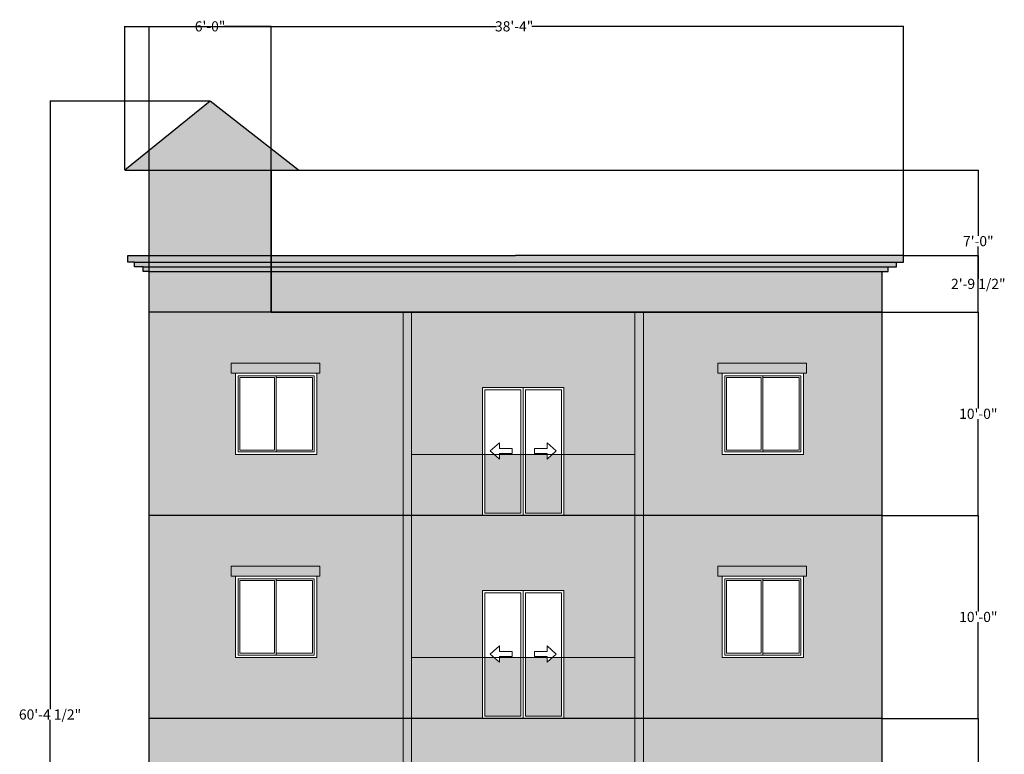
# Model space of a CAD drawing. Units: inches. Extents: x -113 to 5399, y -1393 to 3302.
# Tile 21 of 40: x 3613 to 4195, y -941 to -507. Entities that reach past the tile are written whole.
import ezdxf

# ---------------------------------------------------------------- set-up
doc = ezdxf.new("R2010")
doc.units = ezdxf.units.IN
doc.header["$MEASUREMENT"] = 0
for name, color, linetype, lineweight in [('A-ANNO-DIMS', 254, 'Continuous', 18), ('A-Door', 150, 'Continuous', 18), ('A-ELEV', 7, 'Continuous', 25), ('A-ELEV-GLAZ', 150, 'Continuous', 18), ('A-ELEV-RAIL', 7, 'Continuous', 18), ('A-ELEV-TRIM', 7, 'Continuous', 18), ('A-ELEV-TRIM-PATT', 7, 'Continuous', 13), ('A-ROOF', 7, 'Continuous', 25), ('A-ROOF-CORN-PATT', 3, 'Continuous', 13)]:
    doc.layers.add(name, color=color, linetype=linetype, lineweight=lineweight)
for name, color, linetype, lineweight, true_color in [('A-ELEV-RAIL-PATT', 9, 'Continuous', 13, 0xc7c8ca), ('A-ELEV-WALL-PATT', 241, 'Continuous', 13, 0xf7abae), ('A-ROOF-PATT', 251, 'Continuous', 13, 0x636466)]:
    doc.layers.add(name, color=color, linetype=linetype, lineweight=lineweight, true_color=true_color)
doc.styles.get("Standard").update_dxf_attribs({"font": 'arial.ttf'})
doc.dimstyles.get("Standard").update_dxf_attribs({"dimtxt": 6, "dimasz": 0.18, "dimexe": 0.18, "dimexo": 0.0625, "dimgap": 0.09, "dimtad": 0, "dimtih": 1, "dimtoh": 1, "dimdec": 1, "dimzin": 0, "dimdsep": 46, "dimlunit": 4, "dimtxsty": 'Standard', "dimblk": 'ARCHTICK', "dimcen": 0.09, "dimadec": 0, "dimazin": 0, "dimtfac": 1, "dimtdec": 1, "dimtofl": 0, "dimtmove": 0, "dimatfit": 3, "dimfxl": 1, "dimtolj": 1, "dimtzin": 0, "dimarcsym": 0})

# ---------------------------------------------------------------- blocks, each defined once
blk = doc.blocks.new('*U84')
for p, q in [((1.5, 1.5), (1.5, 46.5)), ((1.5, 46.5), (24, 46.5)), ((24, 1.5), (24, 46.5)), ((24, 46.5), (46.5, 46.5)), ((46.5, 46.5), (46.5, 1.5)), ((24, 1.5), (1.5, 1.5)), ((46.5, 1.5), (24, 1.5))]:
    blk.add_line(p, q)
blk.add_lwpolyline([(0, 0), (0, 48), (48, 48), (48, 0)], close=True)
for points in [[(23, 45.5), (23, 2.5), (2.5, 2.5), (2.5, 45.5), (23, 45.5)], [(24, 45.5), (45.5, 45.5), (45.5, 2.5), (24, 2.5)]]:
    blk.add_lwpolyline(points)
blk = doc.blocks.new('DOOR-SLIDING-PAIR-ELEV')
for p, q in [((9.94, 42.86), (4.53, 38.04)), ((9.94, 39.54), (9.94, 42.86)), ((38.06, 39.54), (38.06, 42.86)), ((38.06, 42.86), (43.47, 38.04)), ((9.94, 33.21), (4.53, 38.04)), ((17.43, 39.54), (9.94, 39.54)), ((17.43, 36.54), (9.94, 36.54)), ((9.94, 36.54), (9.94, 33.21)), ((17.43, 39.54), (17.43, 36.54)), ((30.57, 39.54), (38.06, 39.54)), ((30.57, 39.54), (30.57, 36.54)), ((30.57, 36.54), (38.06, 36.54)), ((38.06, 33.21), (43.47, 38.04)), ((38.06, 36.54), (38.06, 33.21))]:
    blk.add_line(p, q)
for points in [[(0, 75.57), (24, 75.57), (24, 0), (0, 0)], [(1.37, 74.2), (22.63, 74.2), (22.63, 1.37), (1.37, 1.37)], [(24, 75.57), (48, 75.57), (48, 0), (24, 0)], [(25.37, 74.2), (46.63, 74.2), (46.63, 1.37), (25.37, 1.37)]]:
    blk.add_lwpolyline(points, close=True)
blk = doc.blocks.new('_ArchTick')
at = {"color": 0, "linetype": 'ByBlock', "const_width": 0.15}
blk.add_lwpolyline([(-0.5, -0.5), (0.5, 0.5)], dxfattribs=at)
blk = doc.blocks.new('*D213')
at = {"layer": 'A-ANNO-DIMS', "color": 0, "lineweight": -2, "transparency": 16777216}
for p, q in [((3675.33, -596.07), (3675.33, -511.08)), ((3675.33, -511.26), (3894.96, -511.26)), ((4135.38, -511.26), (3915.75, -511.26)), ((4135.38, -646.59), (4135.38, -511.08))]:
    blk.add_line(p, q, dxfattribs=at)
at = {"layer": 'Defpoints', "color": 0, "transparency": 16777216}
for p in [(4135.38, -511.26), (3675.33, -596.13), (4135.38, -646.65)]:
    blk.add_point(p, dxfattribs=at)
at = {"layer": 'A-ANNO-DIMS', "color": 0, "lineweight": -2, "transparency": 16777216, "xscale": 0.18, "yscale": 0.18, "zscale": 0.18, "rotation": 180}
blk.add_blockref('_ArchTick', (3675.33, -511.26), dxfattribs=at)
at = {"layer": 'A-ANNO-DIMS', "color": 0, "lineweight": -2, "transparency": 16777216, "xscale": 0.18, "yscale": 0.18, "zscale": 0.18}
blk.add_blockref('_ArchTick', (4135.38, -511.26), dxfattribs=at)
at = {"layer": 'A-ANNO-DIMS', "color": 0, "transparency": 16777216, "insert": (3905.35, -511.26), "char_height": 6, "attachment_point": 5}
blk.add_mtext('\\A1;38\'-4"', dxfattribs=at)
blk = doc.blocks.new('*D214')
at = {"layer": 'A-ANNO-DIMS', "color": 0, "lineweight": -2, "transparency": 16777216}
for p, q in [((3725.67, -555.41), (3631, -555.41)), ((3631.18, -555.41), (3631.18, -914.58)), ((3631.18, -1280.13), (3631.18, -920.96)), ((3689.67, -1280.13), (3631, -1280.13))]:
    blk.add_line(p, q, dxfattribs=at)
at = {"layer": 'Defpoints', "color": 0, "transparency": 16777216}
for p in [(3631.18, -555.41), (3725.73, -555.41), (3689.73, -1280.13)]:
    blk.add_point(p, dxfattribs=at)
at = {"layer": 'A-ANNO-DIMS', "color": 0, "lineweight": -2, "transparency": 16777216, "xscale": 0.18, "yscale": 0.18, "zscale": 0.18}
for p, rotation in [((3631.18, -555.41), 90), ((3631.18, -1280.13), 270)]:
    blk.add_blockref('_ArchTick', p, dxfattribs=dict(at, rotation=rotation))
at = {"layer": 'A-ANNO-DIMS', "color": 0, "transparency": 16777216, "insert": (3631.18, -917.77), "char_height": 6, "attachment_point": 5}
blk.add_mtext('\\A1;60\'-4 1/2"', dxfattribs=at)
blk = doc.blocks.new('*D223')
at = {"layer": 'A-ANNO-DIMS', "color": 0, "lineweight": -2, "transparency": 16777216}
for p, q in [((4122.79, -920.13), (4179.71, -920.13)), ((4179.53, -920.13), (4179.53, -976.98)), ((4179.53, -1040.13), (4179.53, -983.29)), ((4122.79, -1040.13), (4179.71, -1040.13))]:
    blk.add_line(p, q, dxfattribs=at)
at = {"layer": 'Defpoints', "color": 0, "transparency": 16777216}
for p in [(4122.73, -920.13), (4179.53, -920.13), (4122.73, -1040.13)]:
    blk.add_point(p, dxfattribs=at)
at = {"layer": 'A-ANNO-DIMS', "color": 0, "lineweight": -2, "transparency": 16777216, "xscale": 0.18, "yscale": 0.18, "zscale": 0.18}
for p, rotation in [((4179.53, -920.13), 90), ((4179.53, -1040.13), 270)]:
    blk.add_blockref('_ArchTick', p, dxfattribs=dict(at, rotation=rotation))
at = {"layer": 'A-ANNO-DIMS', "color": 0, "transparency": 16777216, "insert": (4179.53, -980.13), "char_height": 6, "attachment_point": 5}
blk.add_mtext('\\A1;10\'-0"', dxfattribs=at)
blk = doc.blocks.new('*D224')
at = {"layer": 'A-ANNO-DIMS', "color": 0, "lineweight": -2, "transparency": 16777216}
for p, q in [((4122.79, -800.13), (4179.71, -800.13)), ((4179.53, -800.13), (4179.53, -856.98)), ((4179.53, -920.13), (4179.53, -863.29)), ((4122.79, -920.13), (4179.71, -920.13))]:
    blk.add_line(p, q, dxfattribs=at)
at = {"layer": 'Defpoints', "color": 0, "transparency": 16777216}
for p in [(4122.73, -800.13), (4179.53, -800.13), (4122.73, -920.13)]:
    blk.add_point(p, dxfattribs=at)
at = {"layer": 'A-ANNO-DIMS', "color": 0, "lineweight": -2, "transparency": 16777216, "xscale": 0.18, "yscale": 0.18, "zscale": 0.18}
for p, rotation in [((4179.53, -800.13), 90), ((4179.53, -920.13), 270)]:
    blk.add_blockref('_ArchTick', p, dxfattribs=dict(at, rotation=rotation))
at = {"layer": 'A-ANNO-DIMS', "color": 0, "transparency": 16777216, "insert": (4179.53, -860.13), "char_height": 6, "attachment_point": 5}
blk.add_mtext('\\A1;10\'-0"', dxfattribs=at)
blk = doc.blocks.new('*D225')
at = {"layer": 'A-ANNO-DIMS', "color": 0, "lineweight": -2, "transparency": 16777216}
for p, q in [((4122.79, -680.13), (4179.71, -680.13)), ((4179.53, -680.13), (4179.53, -736.98)), ((4179.53, -800.13), (4179.53, -743.29)), ((4122.79, -800.13), (4179.71, -800.13))]:
    blk.add_line(p, q, dxfattribs=at)
at = {"layer": 'Defpoints', "color": 0, "transparency": 16777216}
for p in [(4122.73, -680.13), (4179.53, -680.13), (4122.73, -800.13)]:
    blk.add_point(p, dxfattribs=at)
at = {"layer": 'A-ANNO-DIMS', "color": 0, "lineweight": -2, "transparency": 16777216, "xscale": 0.18, "yscale": 0.18, "zscale": 0.18}
for p, rotation in [((4179.53, -680.13), 90), ((4179.53, -800.13), 270)]:
    blk.add_blockref('_ArchTick', p, dxfattribs=dict(at, rotation=rotation))
at = {"layer": 'A-ANNO-DIMS', "color": 0, "transparency": 16777216, "insert": (4179.53, -740.13), "char_height": 6, "attachment_point": 5}
blk.add_mtext('\\A1;10\'-0"', dxfattribs=at)
blk = doc.blocks.new('*D226')
at = {"layer": 'A-ANNO-DIMS', "color": 0, "lineweight": -2, "transparency": 16777216}
for p, q in [((4135.44, -646.65), (4179.71, -646.65)), ((4179.53, -646.65), (4179.53, -660.2)), ((4179.53, -680.13), (4179.53, -666.59)), ((4122.79, -680.13), (4179.71, -680.13))]:
    blk.add_line(p, q, dxfattribs=at)
at = {"layer": 'Defpoints', "color": 0, "transparency": 16777216}
for p in [(4135.38, -646.65), (4179.53, -646.65), (4122.73, -680.13)]:
    blk.add_point(p, dxfattribs=at)
at = {"layer": 'A-ANNO-DIMS', "color": 0, "lineweight": -2, "transparency": 16777216, "xscale": 0.18, "yscale": 0.18, "zscale": 0.18}
for p, rotation in [((4179.53, -646.65), 90), ((4179.53, -680.13), 270)]:
    blk.add_blockref('_ArchTick', p, dxfattribs=dict(at, rotation=rotation))
at = {"layer": 'A-ANNO-DIMS', "color": 0, "transparency": 16777216, "insert": (4179.53, -663.39), "char_height": 6, "attachment_point": 5}
blk.add_mtext('\\A1;2\'-9 1/2"', dxfattribs=at)
blk = doc.blocks.new('*D227')
at = {"layer": 'A-ANNO-DIMS', "color": 0, "lineweight": -2, "transparency": 16777216}
for p, q in [((3689.73, -680.07), (3689.73, -511.08)), ((3689.73, -511.26), (3717.65, -511.26)), ((3761.73, -511.26), (3733.81, -511.26)), ((3761.73, -680.07), (3761.73, -511.08))]:
    blk.add_line(p, q, dxfattribs=at)
at = {"layer": 'Defpoints', "color": 0, "transparency": 16777216}
for p in [(3761.73, -511.26), (3689.73, -680.13), (3761.73, -680.13)]:
    blk.add_point(p, dxfattribs=at)
at = {"layer": 'A-ANNO-DIMS', "color": 0, "lineweight": -2, "transparency": 16777216, "xscale": 0.18, "yscale": 0.18, "zscale": 0.18, "rotation": 180}
blk.add_blockref('_ArchTick', (3689.73, -511.26), dxfattribs=at)
at = {"layer": 'A-ANNO-DIMS', "color": 0, "lineweight": -2, "transparency": 16777216, "xscale": 0.18, "yscale": 0.18, "zscale": 0.18}
blk.add_blockref('_ArchTick', (3761.73, -511.26), dxfattribs=at)
at = {"layer": 'A-ANNO-DIMS', "color": 0, "transparency": 16777216, "insert": (3725.73, -511.26), "char_height": 6, "attachment_point": 5}
blk.add_mtext('\\A1;6\'-0"', dxfattribs=at)
blk = doc.blocks.new('*D228')
at = {"layer": 'A-ANNO-DIMS', "color": 0, "lineweight": -2, "transparency": 16777216}
for p, q in [((3761.79, -596.13), (4179.71, -596.13)), ((4179.53, -596.13), (4179.53, -634.98)), ((4179.53, -680.13), (4179.53, -641.29)), ((3761.79, -680.13), (4179.71, -680.13))]:
    blk.add_line(p, q, dxfattribs=at)
at = {"layer": 'Defpoints', "color": 0, "transparency": 16777216}
for p in [(3761.73, -596.13), (4179.53, -596.13), (3761.73, -680.13)]:
    blk.add_point(p, dxfattribs=at)
at = {"layer": 'A-ANNO-DIMS', "color": 0, "lineweight": -2, "transparency": 16777216, "xscale": 0.18, "yscale": 0.18, "zscale": 0.18}
for p, rotation in [((4179.53, -596.13), 90), ((4179.53, -680.13), 270)]:
    blk.add_blockref('_ArchTick', p, dxfattribs=dict(at, rotation=rotation))
at = {"layer": 'A-ANNO-DIMS', "color": 0, "transparency": 16777216, "insert": (4179.53, -638.13), "char_height": 6, "attachment_point": 5}
blk.add_mtext('\\A1;7\'-0"', dxfattribs=at)

msp = doc.modelspace()

# ---------------------------------------------------------------- hatches: boundary and pattern name
at = {"layer": 'A-ELEV-RAIL-PATT', "transparency": 33554498}
h = msp.add_hatch(color=256, dxfattribs=at)
h.dxf.hatch_style = 1
h.paths.add_polyline_path([(3886.73, -764.13), (3844.73, -764.13), (3844.73, -800.13), (3886.73, -800.13)])
h.paths.add_polyline_path([(3976.73, -764.13), (3934.73, -764.13), (3934.73, -800.13), (3976.73, -800.13)])
h.paths.add_polyline_path([(3933.36, -764.13), (3927.91, -764.13), (3924.79, -766.92), (3924.79, -764.13), (3912.1, -764.13), (3912.1, -798.76), (3933.36, -798.76)])
h.paths.add_polyline_path([(3909.36, -764.13), (3896.67, -764.13), (3896.67, -766.92), (3893.55, -764.13), (3888.1, -764.13), (3888.1, -798.76), (3909.36, -798.76)])
h = msp.add_hatch(color=256, dxfattribs=at)
h.dxf.hatch_style = 1
h.paths.add_polyline_path([(3886.73, -884.13), (3844.73, -884.13), (3844.73, -920.13), (3886.73, -920.13)])
h.paths.add_polyline_path([(3976.73, -884.13), (3934.73, -884.13), (3934.73, -920.13), (3976.73, -920.13)])
h.paths.add_polyline_path([(3933.36, -884.13), (3927.91, -884.13), (3924.79, -886.92), (3924.79, -884.13), (3912.1, -884.13), (3912.1, -918.76), (3933.36, -918.76)])
h.paths.add_polyline_path([(3909.36, -884.13), (3896.67, -884.13), (3896.67, -886.92), (3893.55, -884.13), (3888.1, -884.13), (3888.1, -918.76), (3909.36, -918.76)])
at = {"layer": 'A-ELEV-TRIM-PATT'}
h = msp.add_hatch(color=256, dxfattribs=at)
h.dxf.hatch_style = 1
h.paths.add_polyline_path([(4122.73, -656.13), (3689.73, -656.13), (3689.73, -680.13), (4122.73, -680.13)])
h = msp.add_hatch(color=256, dxfattribs=at)
h.dxf.hatch_style = 1
h.paths.add_polyline_path([(3981.73, -1040.13), (3976.73, -1040.13), (3976.73, -1160.13), (3981.73, -1160.13)])
h.paths.add_polyline_path([(3981.73, -920.13), (3976.73, -920.13), (3976.73, -1040.13), (3981.73, -1040.13)])
h.paths.add_polyline_path([(3981.73, -800.13), (3976.73, -800.13), (3976.73, -920.13), (3981.73, -920.13)])
h.paths.add_polyline_path([(3981.73, -680.13), (3976.73, -680.13), (3976.73, -800.13), (3981.73, -800.13)])
h.paths.add_polyline_path([(3844.73, -680.13), (3839.73, -680.13), (3839.73, -800.13), (3844.73, -800.13)])
h.paths.add_polyline_path([(3844.73, -800.13), (3839.73, -800.13), (3839.73, -920.13), (3844.73, -920.13)])
h.paths.add_polyline_path([(3844.73, -920.13), (3839.73, -920.13), (3839.73, -1040.13), (3844.73, -1040.13)])
h.paths.add_polyline_path([(3844.73, -1040.13), (3839.73, -1040.13), (3839.73, -1160.13), (3844.73, -1160.13)])
h = msp.add_hatch(color=256, dxfattribs=at)
h.dxf.hatch_style = 1
h.paths.add_polyline_path([(4078.05, -1190.14), (4025.64, -1190.14), (4025.64, -1196.13), (4078.05, -1196.13)])
h.paths.add_polyline_path([(3790.55, -1190.14), (3738.14, -1190.14), (3738.14, -1196.13), (3790.55, -1196.13)])
h.paths.add_polyline_path([(3790.55, -1070.14), (3738.14, -1070.14), (3738.14, -1076.13), (3790.55, -1076.13)])
h.paths.add_polyline_path([(3790.55, -950.14), (3738.14, -950.14), (3738.14, -956.13), (3790.55, -956.13)])
h.paths.add_polyline_path([(3790.55, -830.14), (3738.14, -830.14), (3738.14, -836.13), (3790.55, -836.13)])
h.paths.add_polyline_path([(4078.05, -830.14), (4025.64, -830.14), (4025.64, -836.13), (4078.05, -836.13)])
h.paths.add_polyline_path([(4078.05, -710.14), (4025.64, -710.14), (4025.64, -716.13), (4078.05, -716.13)])
h.paths.add_polyline_path([(3790.55, -710.14), (3738.14, -710.14), (3738.14, -716.13), (3790.55, -716.13)])
h.paths.add_polyline_path([(4078.05, -1070.14), (4025.64, -1070.14), (4025.64, -1076.13), (4078.05, -1076.13)])
h.paths.add_polyline_path([(4078.05, -950.14), (4025.64, -950.14), (4025.64, -956.13), (4078.05, -956.13)])
at = {"layer": 'A-ELEV-WALL-PATT'}
h = msp.add_hatch(color=256, dxfattribs=at)
h.dxf.hatch_style = 1
h.paths.add_polyline_path([(3761.73, -596.13), (3689.73, -596.13), (3689.73, -680.13), (3761.73, -680.13)])
h = msp.add_hatch(color=256, dxfattribs=at)
h.dxf.hatch_style = 1
h.paths.add_polyline_path([(3839.73, -680.13), (3689.73, -680.13), (3689.73, -800.13), (3839.73, -800.13)])
h.paths.add_polyline_path([(3790.55, -716.13), (3788.73, -716.13), (3788.73, -764.13), (3740.73, -764.13), (3740.73, -716.13), (3738.14, -716.13), (3738.14, -710.14), (3790.55, -710.14)], flags=16)
h.paths.add_polyline_path([(3787.23, -717.63), (3787.23, -762.63), (3764.73, -762.63), (3742.23, -762.63), (3742.23, -717.63), (3764.73, -717.63)], flags=0)
h.paths.add_polyline_path([(3786.23, -718.63), (3786.23, -761.63), (3764.73, -761.63), (3764.73, -718.63)], flags=0)
h.paths.add_polyline_path([(3763.73, -761.63), (3743.23, -761.63), (3743.23, -718.63), (3763.73, -718.63)], flags=0)
h.paths.add_polyline_path([(3976.73, -680.13), (3844.73, -680.13), (3844.73, -764.13), (3886.73, -764.13), (3886.73, -724.56), (3910.73, -724.56), (3934.73, -724.56), (3934.73, -764.13), (3976.73, -764.13)])
h.paths.add_polyline_path([(4122.73, -680.13), (3981.73, -680.13), (3981.73, -800.13), (4122.73, -800.13)])
h.paths.add_polyline_path([(4028.23, -716.13), (4025.64, -716.13), (4025.64, -710.14), (4078.05, -710.14), (4078.05, -716.13), (4076.23, -716.13), (4076.23, -764.13), (4028.23, -764.13)], flags=16)
h.paths.add_polyline_path([(4029.73, -717.63), (4052.23, -717.63), (4074.73, -717.63), (4074.73, -762.63), (4052.23, -762.63), (4029.73, -762.63)], flags=0)
h.paths.add_polyline_path([(4030.73, -718.63), (4051.23, -718.63), (4051.23, -761.63), (4030.73, -761.63)], flags=0)
h.paths.add_polyline_path([(4052.23, -718.63), (4073.73, -718.63), (4073.73, -761.63), (4052.23, -761.63)], flags=0)
h.paths.add_polyline_path([(4122.73, -800.13), (3981.73, -800.13), (3981.73, -920.13), (4122.73, -920.13)])
h.paths.add_polyline_path([(4025.64, -836.13), (4025.64, -830.14), (4078.05, -830.14), (4078.05, -836.13), (4076.23, -836.13), (4076.23, -884.13), (4028.23, -884.13), (4028.23, -836.13)], flags=16)
h.paths.add_polyline_path([(4029.73, -837.63), (4052.23, -837.63), (4074.73, -837.63), (4074.73, -882.63), (4052.23, -882.63), (4029.73, -882.63)], flags=0)
h.paths.add_polyline_path([(4030.73, -838.63), (4051.23, -838.63), (4051.23, -881.63), (4030.73, -881.63)], flags=0)
h.paths.add_polyline_path([(4052.23, -838.63), (4073.73, -838.63), (4073.73, -881.63), (4052.23, -881.63)], flags=0)
h.paths.add_polyline_path([(3976.73, -800.13), (3844.73, -800.13), (3844.73, -884.13), (3886.73, -884.13), (3886.73, -844.56), (3910.73, -844.56), (3934.73, -844.56), (3934.73, -884.13), (3976.73, -884.13)])
h.paths.add_polyline_path([(3839.73, -800.13), (3689.73, -800.13), (3689.73, -920.13), (3839.73, -920.13)])
h.paths.add_polyline_path([(3788.73, -884.13), (3740.73, -884.13), (3740.73, -836.13), (3738.14, -836.13), (3738.14, -830.14), (3790.55, -830.14), (3790.55, -836.13), (3788.73, -836.13)], flags=16)
h.paths.add_polyline_path([(3787.23, -882.63), (3764.73, -882.63), (3742.23, -882.63), (3742.23, -837.63), (3764.73, -837.63), (3787.23, -837.63)], flags=0)
h.paths.add_polyline_path([(3786.23, -881.63), (3764.73, -881.63), (3764.73, -838.63), (3786.23, -838.63)], flags=0)
h.paths.add_polyline_path([(3763.73, -881.63), (3743.23, -881.63), (3743.23, -838.63), (3763.73, -838.63)], flags=0)
h.paths.add_polyline_path([(3839.73, -920.13), (3689.73, -920.13), (3689.73, -1040.13), (3839.73, -1040.13)])
h.paths.add_polyline_path([(3788.73, -1004.13), (3740.73, -1004.13), (3740.73, -956.13), (3738.14, -956.13), (3738.14, -950.14), (3790.55, -950.14), (3790.55, -956.13), (3788.73, -956.13)], flags=16)
h.paths.add_polyline_path([(3787.23, -1002.63), (3764.73, -1002.63), (3742.23, -1002.63), (3742.23, -957.63), (3764.73, -957.63), (3787.23, -957.63)], flags=0)
h.paths.add_polyline_path([(3786.23, -1001.63), (3764.73, -1001.63), (3764.73, -958.63), (3786.23, -958.63)], flags=0)
h.paths.add_polyline_path([(3763.73, -1001.63), (3743.23, -1001.63), (3743.23, -958.63), (3763.73, -958.63)], flags=0)
h.paths.add_polyline_path([(3976.73, -920.13), (3844.73, -920.13), (3844.73, -1004.13), (3886.73, -1004.13), (3886.73, -964.56), (3910.73, -964.56), (3934.73, -964.56), (3934.73, -1004.13), (3976.73, -1004.13)])
h.paths.add_polyline_path([(4122.73, -920.13), (3981.73, -920.13), (3981.73, -1040.13), (4122.73, -1040.13)])
h.paths.add_polyline_path([(4028.23, -956.13), (4025.64, -956.13), (4025.64, -950.14), (4078.05, -950.14), (4078.05, -956.13), (4076.23, -956.13), (4076.23, -1004.13), (4028.23, -1004.13)], flags=16)
h.paths.add_polyline_path([(4029.73, -957.63), (4052.23, -957.63), (4074.73, -957.63), (4074.73, -1002.63), (4052.23, -1002.63), (4029.73, -1002.63)], flags=0)
h.paths.add_polyline_path([(4030.73, -958.63), (4051.23, -958.63), (4051.23, -1001.63), (4030.73, -1001.63)], flags=0)
h.paths.add_polyline_path([(4052.23, -958.63), (4073.73, -958.63), (4073.73, -1001.63), (4052.23, -1001.63)], flags=0)
h.paths.add_polyline_path([(4122.73, -1040.13), (3981.73, -1040.13), (3981.73, -1160.13), (4122.73, -1160.13)])
h.paths.add_polyline_path([(4028.23, -1076.13), (4025.64, -1076.13), (4025.64, -1070.14), (4078.05, -1070.14), (4078.05, -1076.13), (4076.23, -1076.13), (4076.23, -1124.13), (4028.23, -1124.13)], flags=16)
h.paths.add_polyline_path([(4029.73, -1077.63), (4052.23, -1077.63), (4074.73, -1077.63), (4074.73, -1122.63), (4052.23, -1122.63), (4029.73, -1122.63)], flags=0)
h.paths.add_polyline_path([(4030.73, -1078.63), (4051.23, -1078.63), (4051.23, -1121.63), (4030.73, -1121.63)], flags=0)
h.paths.add_polyline_path([(4052.23, -1078.63), (4073.73, -1078.63), (4073.73, -1121.63), (4052.23, -1121.63)], flags=0)
h.paths.add_polyline_path([(3976.73, -1040.13), (3844.73, -1040.13), (3844.73, -1124.13), (3886.73, -1124.13), (3886.73, -1084.56), (3910.73, -1084.56), (3934.73, -1084.56), (3934.73, -1124.13), (3976.73, -1124.13)])
h.paths.add_polyline_path([(3839.73, -1040.13), (3689.73, -1040.13), (3689.73, -1160.13), (3839.73, -1160.13)])
h.paths.add_polyline_path([(3788.73, -1124.13), (3740.73, -1124.13), (3740.73, -1076.13), (3738.14, -1076.13), (3738.14, -1070.14), (3790.55, -1070.14), (3790.55, -1076.13), (3788.73, -1076.13)], flags=16)
h.paths.add_polyline_path([(3787.23, -1122.63), (3764.73, -1122.63), (3742.23, -1122.63), (3742.23, -1077.63), (3764.73, -1077.63), (3787.23, -1077.63)], flags=0)
h.paths.add_polyline_path([(3786.23, -1121.63), (3764.73, -1121.63), (3764.73, -1078.63), (3786.23, -1078.63)], flags=0)
h.paths.add_polyline_path([(3763.73, -1121.63), (3743.23, -1121.63), (3743.23, -1078.63), (3763.73, -1078.63)], flags=0)
h.paths.add_polyline_path([(3886.73, -1208.13), (3934.73, -1208.13), (3934.73, -1280.13), (4122.73, -1280.13), (4122.73, -1160.13), (3981.73, -1160.13), (3689.73, -1160.13), (3689.73, -1280.13), (3886.73, -1280.13)])
h.paths.add_polyline_path([(3788.73, -1244.13), (3740.73, -1244.13), (3740.73, -1196.13), (3738.14, -1196.13), (3738.14, -1190.14), (3790.55, -1190.14), (3790.55, -1196.13), (3788.73, -1196.13)], flags=16)
h.paths.add_polyline_path([(3787.23, -1242.63), (3764.73, -1242.63), (3742.23, -1242.63), (3742.23, -1197.63), (3764.73, -1197.63), (3787.23, -1197.63)], flags=0)
h.paths.add_polyline_path([(3786.23, -1241.63), (3764.73, -1241.63), (3764.73, -1198.63), (3786.23, -1198.63)], flags=0)
h.paths.add_polyline_path([(3763.73, -1241.63), (3743.23, -1241.63), (3743.23, -1198.63), (3763.73, -1198.63)], flags=0)
h.paths.add_polyline_path([(4025.64, -1196.13), (4025.64, -1190.14), (4078.05, -1190.14), (4078.05, -1196.13), (4076.23, -1196.13), (4076.23, -1244.13), (4028.23, -1244.13), (4028.23, -1196.13)], flags=16)
h.paths.add_polyline_path([(4029.73, -1197.63), (4052.23, -1197.63), (4074.73, -1197.63), (4074.73, -1242.63), (4052.23, -1242.63), (4029.73, -1242.63)], flags=0)
h.paths.add_polyline_path([(4030.73, -1198.63), (4051.23, -1198.63), (4051.23, -1241.63), (4030.73, -1241.63)], flags=0)
h.paths.add_polyline_path([(4052.23, -1198.63), (4073.73, -1198.63), (4073.73, -1241.63), (4052.23, -1241.63)], flags=0)
at = {"layer": 'A-ROOF-CORN-PATT'}
h = msp.add_hatch(color=256, dxfattribs=at)
h.dxf.hatch_style = 1
h.paths.add_polyline_path([(4135.38, -646.65), (3906.23, -646.65), (3677.08, -646.65), (3677.08, -650.56), (3681.16, -650.56), (4131.3, -650.56), (4135.38, -650.56)])
h.paths.add_polyline_path([(4131.3, -650.56), (3681.16, -650.56), (3681.16, -653.25), (3686.21, -653.25), (4126.25, -653.25), (4131.3, -653.25)])
h.paths.add_polyline_path([(4126.25, -653.25), (3686.21, -653.25), (3686.21, -656.13), (3689.73, -656.13), (4122.73, -656.13), (4126.25, -656.13)])
at = {"layer": 'A-ROOF-PATT'}
h = msp.add_hatch(color=256, dxfattribs=at)
h.dxf.hatch_style = 1
h.paths.add_polyline_path([(3725.73, -555.41), (3675.33, -596.13), (3689.73, -596.13), (3761.73, -596.13), (3778, -596.13)])

# ---------------------------------------------------------------- linework, layer by layer
at = {"layer": 'A-ELEV'}
for p, q in [((3689.73, -800.13), (3689.73, -680.13)), ((4122.73, -680.13), (3689.73, -680.13)), ((4122.73, -800.13), (4122.73, -680.13)), ((4122.73, -800.13), (4122.73, -680.13)), ((3689.73, -920.13), (3689.73, -800.13)), ((4122.73, -800.13), (3689.73, -800.13)), ((4122.73, -920.13), (4122.73, -800.13)), ((4122.73, -920.13), (4122.73, -800.13)), ((3689.73, -1040.13), (3689.73, -920.13)), ((4122.73, -920.13), (3689.73, -920.13)), ((4122.73, -1040.13), (4122.73, -920.13)), ((4122.73, -1040.13), (4122.73, -920.13))]:
    msp.add_line(p, q, dxfattribs=at)
at = {"layer": 'A-ELEV-GLAZ'}
for p, q in [((3740.73, -764.13), (3740.73, -716.13)), ((3788.73, -764.13), (3788.73, -716.13)), ((4028.23, -764.13), (4028.23, -716.13)), ((4076.23, -764.13), (4076.23, -716.13)), ((3740.73, -884.13), (3740.73, -836.13)), ((3788.73, -884.13), (3788.73, -836.13)), ((4028.23, -884.13), (4028.23, -836.13)), ((4076.23, -884.13), (4076.23, -836.13))]:
    msp.add_line(p, q, dxfattribs=at)
at = {"layer": 'A-ELEV-RAIL'}
for p, q in [((3844.73, -764.13), (3976.73, -764.13)), ((3844.73, -884.13), (3976.73, -884.13))]:
    msp.add_line(p, q, dxfattribs=at)
at = {"layer": 'A-ELEV-TRIM'}
for p, q in [((3839.73, -800.13), (3839.73, -680.13)), ((3844.73, -800.13), (3844.73, -680.13)), ((3976.73, -800.13), (3976.73, -680.13)), ((3981.73, -800.13), (3981.73, -680.13)), ((3839.73, -920.13), (3839.73, -800.13)), ((3844.73, -920.13), (3844.73, -800.13)), ((3976.73, -920.13), (3976.73, -800.13)), ((3981.73, -920.13), (3981.73, -800.13)), ((3839.73, -1040.13), (3839.73, -920.13)), ((3844.73, -1040.13), (3844.73, -920.13)), ((3976.73, -1040.13), (3976.73, -920.13)), ((3981.73, -1040.13), (3981.73, -920.13))]:
    msp.add_line(p, q, dxfattribs=at)
for points in [[(3738.14, -716.13), (3790.55, -716.13), (3790.55, -710.14), (3738.14, -710.14)], [(4025.64, -716.13), (4078.05, -716.13), (4078.05, -710.14), (4025.64, -710.14)], [(3738.14, -836.13), (3790.55, -836.13), (3790.55, -830.14), (3738.14, -830.14)], [(4025.64, -836.13), (4078.05, -836.13), (4078.05, -830.14), (4025.64, -830.14)]]:
    msp.add_lwpolyline(points, close=True, dxfattribs=at)
at = {"layer": 'A-ROOF'}
for p, q in [((3725.73, -555.41), (3675.33, -596.13)), ((3778, -596.13), (3725.73, -555.41)), ((3675.33, -596.13), (3689.73, -596.13)), ((3689.73, -680.13), (3689.73, -596.13)), ((3689.73, -596.13), (3761.73, -596.13)), ((3761.73, -596.13), (3761.73, -680.13)), ((3761.73, -596.13), (3778, -596.13)), ((3677.08, -650.56), (3677.08, -646.65)), ((3677.08, -646.65), (3906.23, -646.65)), ((3681.16, -650.56), (3677.08, -650.56)), ((3681.16, -653.25), (3681.16, -650.56)), ((3681.16, -650.56), (4131.3, -650.56)), ((4135.38, -646.65), (3906.23, -646.65)), ((4131.3, -653.25), (4131.3, -650.56)), ((4131.3, -650.56), (4135.38, -650.56)), ((4135.38, -650.56), (4135.38, -646.65)), ((3686.21, -653.25), (3681.16, -653.25)), ((3686.21, -656.13), (3686.21, -653.25)), ((3686.21, -653.25), (4126.25, -653.25)), ((3689.73, -656.13), (3686.21, -656.13)), ((3689.73, -680.13), (3689.73, -656.13)), ((3689.73, -656.13), (4122.73, -656.13)), ((4122.73, -680.13), (4122.73, -656.13)), ((4122.73, -656.13), (4126.25, -656.13)), ((4126.25, -656.13), (4126.25, -653.25)), ((4126.25, -653.25), (4131.3, -653.25))]:
    msp.add_line(p, q, dxfattribs=at)

# ---------------------------------------------------------------- block references
at = {"layer": 'A-Door'}
for p in [(3886.73, -800.13), (3886.73, -920.13)]:
    msp.add_blockref('DOOR-SLIDING-PAIR-ELEV', p, dxfattribs=at)
at = {"layer": 'A-ELEV-GLAZ'}
for p in [(3740.73, -764.13), (4028.23, -764.13), (3740.73, -884.13), (4028.23, -884.13)]:
    msp.add_blockref('*U84', p, dxfattribs=at)

# ---------------------------------------------------------------- dimensions: what is measured, and where the dimension line sits
at = {"layer": 'A-ANNO-DIMS'}
for base, p1, p2, picture, middle in [((4135.3795, -511.2607), (3675.325, -596.1334), (4135.3795, -646.6523), '*D213', (3905.3523, -511.2607)), ((3761.73, -511.26), (3689.73, -680.13), (3761.73, -680.13), '*D227', (3725.73, -511.26))]:
    dim = msp.add_linear_dim(base=base, p1=p1, p2=p2, dimstyle='Standard', override={"dimdec": 1, "dimlfac": 1, "dimrnd": 0, "dimzin": 1, "dimdsep": 46, "dimlunit": 4, "dimfrac": 2}, dxfattribs=at)
    dim.commit()
    dim.dimension.update_dxf_attribs({"geometry": picture, "text_midpoint": middle})
for base, p1, p2, picture, middle in [((3631.18, -555.41), (3689.73, -1280.13), (3725.73, -555.41), '*D214', (3631.18, -917.77)), ((4179.53, -596.13), (3761.73, -680.13), (3761.73, -596.13), '*D228', (4179.53, -638.13)), ((4179.53, -646.65), (4122.73, -680.13), (4135.38, -646.65), '*D226', (4179.53, -663.39)), ((4179.53, -680.13), (4122.73, -800.13), (4122.73, -680.13), '*D225', (4179.53, -740.13)), ((4179.53, -800.13), (4122.73, -920.13), (4122.73, -800.13), '*D224', (4179.53, -860.13)), ((4179.53, -920.13), (4122.73, -1040.13), (4122.73, -920.13), '*D223', (4179.53, -980.13))]:
    dim = msp.add_linear_dim(base=base, p1=p1, p2=p2, angle=90, dimstyle='Standard', override={"dimdec": 1, "dimlfac": 1, "dimrnd": 0, "dimzin": 1, "dimdsep": 46, "dimlunit": 4, "dimfrac": 2}, dxfattribs=at)
    dim.commit()
    dim.dimension.update_dxf_attribs({"geometry": picture, "text_midpoint": middle})

doc.saveas('drawing.dxf')
